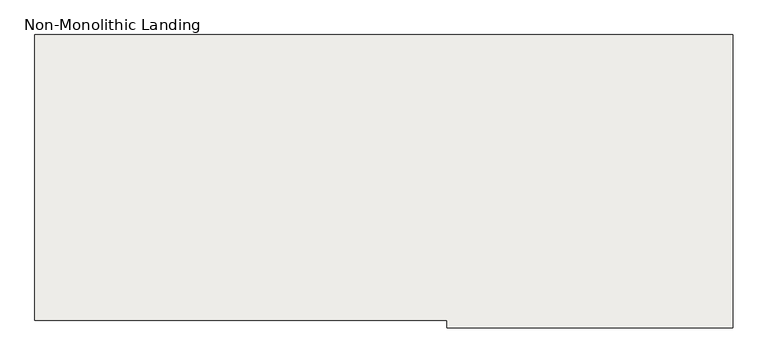
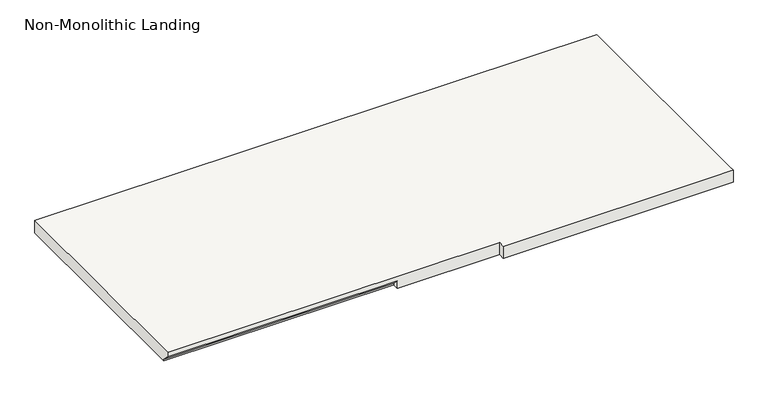
"""IFC4 building model written with IfcOpenShell, lengths in millimetres: slab geometry, Non-Monolithic Landing."""

from ifc_helpers import new_model, si_unit, origin, place, context, project, spatial, faceted_brep, source, transform, mapped, element, save


def non_monolithic_landing_5b8191bc(model_context):
    return source(origin(), model_context, "Body", "Brep", [
        faceted_brep([(-3617.4415084, -19522.1851539, 30634.2339133), (-3617.4415084, -19496.7851539, 30608.8339133), (-2703.0415084, -19496.7851539, 30608.8339133), (-2703.0415084, -19522.1851539, 30634.2339133), (-2296.6415084, -19522.1851539, 30653.2839133), (-2296.6415084, -19547.5851539, 30653.2839133), (-1382.2415084, -19547.5851539, 30653.2839133), (-1382.2415084, -19522.1851539, 30653.2839133), (-1382.2415084, -18607.7851539, 30653.2839133), (-3617.4415084, -18607.7851539, 30653.2839133), (-3617.4415084, -19522.1851539, 30653.2839133), (-2703.0415084, -19496.7851539, 30602.4839133), (-3617.4415084, -19496.7851539, 30602.4839133), (-3617.4415084, -18607.7851539, 30602.4839133), (-1382.2415084, -18607.7851539, 30602.4839133), (-1382.2415084, -19522.1851539, 30602.4839133), (-1382.2415084, -19547.5851539, 30602.4839133), (-2296.6415084, -19547.5851539, 30602.4839133), (-2296.6415084, -19522.1851539, 30602.4839133), (-2703.0415084, -19522.1851539, 30602.4839133)], [[[0, 1, 2, 3]], [[4, 5, 6, 7, 8, 9, 10]], [[11, 12, 13, 14, 15, 16, 17, 18, 19]], [[12, 11, 2, 1]], [[11, 19, 3, 2]], [[4, 10, 0, 3, 19, 18]], [[5, 4, 18, 17]], [[6, 5, 17, 16]], [[7, 6, 16, 15]], [[8, 7, 15, 14]], [[9, 8, 14, 13]], [[10, 9, 13, 12, 1, 0]]]),
    ])


if __name__ == "__main__":
    model = new_model("IFC4")
    model_context = context("Model", 3, world=origin())
    ifc_project = project(units=[si_unit("LENGTHUNIT", "METRE", prefix="MILLI")], contexts=[model_context])
    site = spatial("IfcSite", under=ifc_project)
    building = spatial("IfcBuilding", under=site)
    placement = place(None, origin())
    non_monolithic_landing_shape = non_monolithic_landing_5b8191bc(model_context)
    element("IfcSlab", 1, ObjectType="Non-Monolithic Landing", at=placement, inside=building, context=model_context, shape_type="MappedRepresentation", body=[
        mapped(non_monolithic_landing_shape, transform((0.0, 0.0, 0.0), x_axis=(1.0, 0.0, 0.0), y_axis=(0.0, 1.0, 0.0), z_axis=(0.0, 0.0, 1.0))),
    ])
    save(model, "model.ifc")
